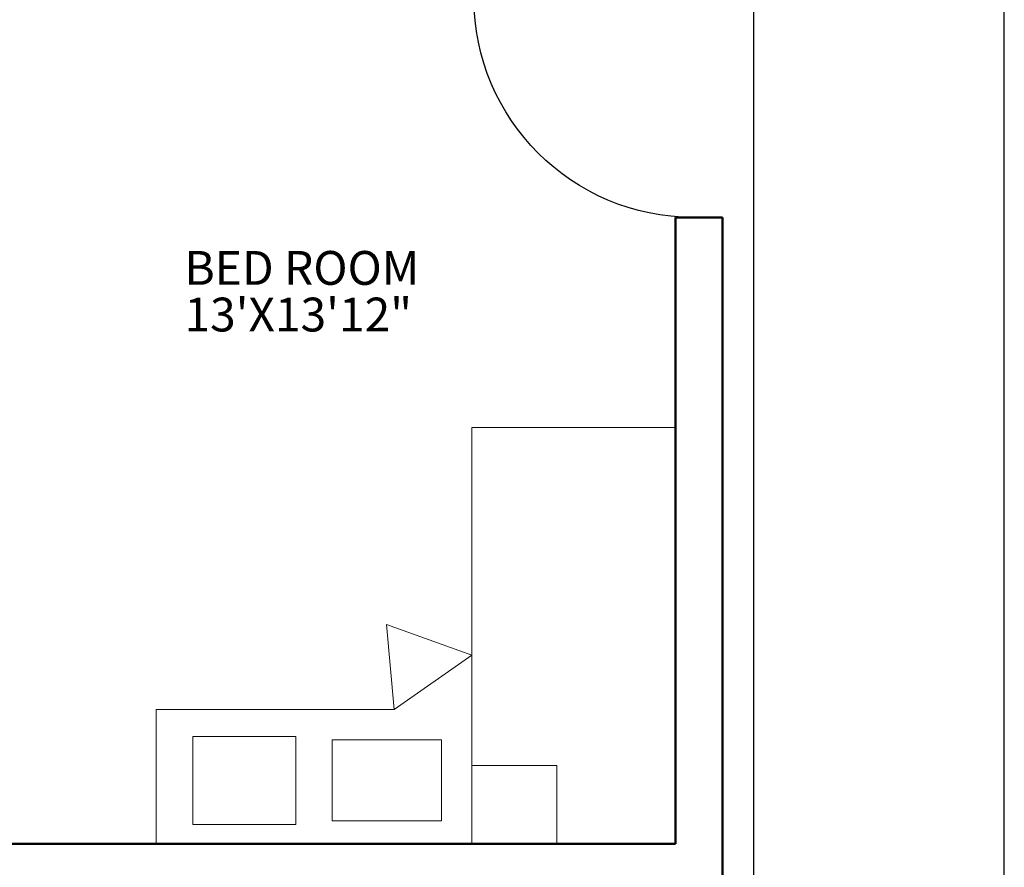
# Model space of a CAD drawing. Units: inches. Extents: x 5375 to 6084, y 16106 to 17259.
# Tile 17 of 32: x 5573 to 5762, y 16518 to 16680. Entities that reach past the tile are written whole.
import ezdxf

# ---------------------------------------------------------------- set-up
doc = ezdxf.new("R2010")
doc.units = ezdxf.units.IN
for name, color, linetype, lineweight in [('A-ANNO-DIMS', 2, 'Continuous', 18), ('A-AREA-IDEN', 5, 'Continuous', 18), ('DOOR', 4, 'Continuous', 25), ('FURNITURE', 3, 'Continuous', 18), ('WALL', 6, 'Continuous', 50)]:
    doc.layers.add(name, color=color, linetype=linetype, lineweight=lineweight)
doc.styles.get("Standard").update_dxf_attribs({"font": 'arial.ttf'})
doc.dimstyles.get("Standard").update_dxf_attribs({"dimtxt": 0.18, "dimasz": 0.18, "dimexe": 0.18, "dimexo": 0.0625, "dimgap": 0.09, "dimtad": 0, "dimtih": 1, "dimtoh": 1, "dimdec": 4, "dimzin": 0, "dimdsep": 46, "dimtxsty": 'Standard', "dimcen": 0.09, "dimadec": 0, "dimazin": 0, "dimtfac": 1, "dimtdec": 4, "dimtofl": 0, "dimtmove": 0, "dimatfit": 3, "dimfxl": 1, "dimtolj": 1, "dimtzin": 0, "dimarcsym": 0})

# ---------------------------------------------------------------- blocks, each defined once
blk = doc.blocks.new('*U2')
for p, q in [((0, 0), (0, -100)), ((750, 0), (750, -100))]:
    blk.add_line(p, q)
blk.add_lwpolyline([(0, 0), (0, 750), (43.75, 750), (43.75, 0)], close=True)
blk.add_arc((0, 0), 750, 0, 90)
blk = doc.blocks.new('*D39')
at = {"layer": 'A-ANNO-DIMS', "color": 0, "lineweight": -2, "transparency": 16777216}
for p, q in [((5713.62, 16402.64), (5713.62, 17259.16)), ((5713.8, 17258.98), (5737.4, 17258.98)), ((5761.44, 17258.98), (5737.84, 17258.98)), ((5761.62, 16402.64), (5761.62, 17259.16))]:
    blk.add_line(p, q, dxfattribs=at)
at = {"layer": 'A-ANNO-DIMS', "color": 0, "transparency": 16777216}
for points in [[(5713.8, 17259.01), (5713.8, 17258.95), (5713.62, 17258.98)], [(5761.44, 17259.01), (5761.44, 17258.95), (5761.62, 17258.98)]]:
    blk.add_solid(points, dxfattribs=at)
at = {"layer": 'Defpoints', "color": 0, "transparency": 16777216}
for p in [(5761.62, 17258.98), (5713.62, 16402.58), (5761.62, 16402.58)]:
    blk.add_point(p, dxfattribs=at)
at = {"layer": 'A-ANNO-DIMS', "color": 0, "transparency": 16777216, "insert": (5737.62, 17258.98), "char_height": 0.18, "attachment_point": 5}
blk.add_mtext('\\A1;48', dxfattribs=at)

msp = doc.modelspace()

# ---------------------------------------------------------------- linework, layer by layer
at = {"layer": 'FURNITURE'}
for p, q in [((5644.722, 16548.3343), (5643.262, 16564.5677)), ((5643.262, 16564.5677), (5659.6045, 16558.7312)), ((5644.722, 16548.3343), (5659.6045, 16558.7312)), ((5644.722, 16548.3343), (5599.1413, 16548.3343)), ((5599.1413, 16548.3343), (5599.1413, 16522.5793))]:
    msp.add_line(p, q, dxfattribs=at)
for points in [[(5698.6199, 16602.3237), (5659.6045, 16602.3237), (5659.6045, 16522.5793), (5698.6199, 16522.5793)], [(5606.1897, 16543.1366), (5625.9169, 16543.1366), (5625.9169, 16526.259), (5606.1897, 16526.259)], [(5632.8547, 16542.4748), (5653.8298, 16542.4748), (5653.8298, 16526.9901), (5632.8547, 16526.9901)], [(5659.6045, 16537.5646), (5675.9133, 16537.5646), (5675.9133, 16522.5793), (5659.6045, 16522.5793)]]:
    msp.add_lwpolyline(points, close=True, dxfattribs=at)
at = {"layer": 'WALL'}
for p, q in [((5707.6199, 16642.5793), (5698.6199, 16642.5793)), ((5698.6199, 16642.5793), (5698.6199, 16522.5793)), ((5707.6199, 16642.5793), (5707.6199, 16507.5793)), ((5536.6199, 16522.5793), (5698.6199, 16522.5793))]:
    msp.add_line(p, q, dxfattribs=at)

# ---------------------------------------------------------------- block references
at = {"layer": 'DOOR', "xscale": -0.0559999999999998, "yscale": 0.0559999999999998, "zscale": 0.0559999999999998, "rotation": 90}
msp.add_blockref('*U2', (5702.0199, 16684.5793), dxfattribs=at)

# ---------------------------------------------------------------- texts
at = {"layer": 'A-AREA-IDEN'}
for s, p in [('BED ROOM', (5604.5531, 16629.6522)), ('13\'X13\'12"', (5604.5531, 16620.7191))]:
    msp.add_text(s, height=6.47981, dxfattribs=at).set_placement(p)

# ---------------------------------------------------------------- dimensions: what is measured, and where the dimension line sits
at = {"layer": 'A-ANNO-DIMS'}
dim = msp.add_linear_dim(base=(5761.6199, 17258.9793), p1=(5713.6199, 16402.5793), p2=(5761.6199, 16402.5793), dimstyle='Standard', override={"dimdec": 0, "dimlfac": 1, "dimrnd": 0, "dimzin": 0, "dimdsep": 46, "dimlunit": 2}, dxfattribs=at)
dim.commit()
dim.dimension.update_dxf_attribs({"geometry": '*D39', "text_midpoint": (5737.6199, 17258.9793)})

doc.saveas('drawing.dxf')
